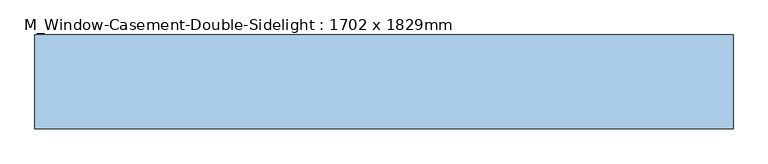
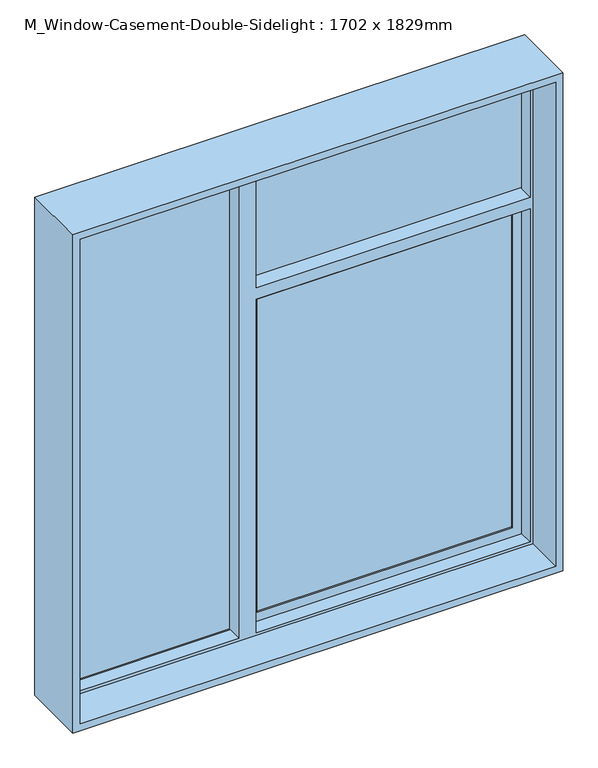
"""IFC4 building model written with IfcOpenShell, lengths in millimetres: window geometry, M_Window-Casement-Double-Sidelight : 1702 x 1829mm."""

from ifc_helpers import new_model, si_unit, frame, origin, place, context, project, spatial, polyline, outline, extrude, faceted_brep, source, transform, mapped, element, save


def m_window_casement_double_sidelight_1702_x_1829mm_c8b42c7f(model_context):
    return source(origin(), model_context, "Body", "SolidModel", [
        extrude(outline(polyline([(783.5796875, 98.4), (-102.8596875, 98.4), (-102.8596875, 111.1), (783.5796875, 111.1), (783.5796875, 98.4)])), frame((0.0, 0.0, 967.3203125), z_axis=(0.0, 0.0, 1.0), x_axis=(1.0, 0.0, 0.0)), (0.0, 0.0, 1.0), 1149.9592187),
        extrude(outline(polyline([(783.5796875, 85.7), (783.5796875, 79.35), (-102.8596875, 79.35), (-102.8596875, 85.7), (783.5796875, 85.7)])), frame((0.0, 0.0, 967.3203125), z_axis=(0.0, 0.0, 1.0), x_axis=(1.0, 0.0, 0.0)), (0.0, 0.0, 1.0), 1149.9592187),
        extrude(outline(polyline([(-195.58, 98.4), (-195.58, 92.05), (-825.5, 92.05), (-825.5, 98.4), (-195.58, 98.4)])), frame((0.0, 0.0, 935.5203125), z_axis=(0.0, 0.0, 1.0), x_axis=(1.0, 0.0, 0.0)), (0.0, 0.0, 1.0), 1767.8796875),
        extrude(outline(polyline([(-195.58, 85.7), (-195.58, 79.35), (-825.5, 79.35), (-825.5, 85.7), (-195.58, 85.7)])), frame((0.0, 0.0, 935.5203125), z_axis=(0.0, 0.0, 1.0), x_axis=(1.0, 0.0, 0.0)), (0.0, 0.0, 1.0), 1767.8796875),
        extrude(outline(polyline([(825.5, 85.7), (825.5, 79.35), (-144.78, 79.35), (-144.78, 85.7), (825.5, 85.7)])), frame((0.0, 0.0, 2201.1201563), z_axis=(0.0, 0.0, 1.0), x_axis=(1.0, 0.0, 0.0)), (0.0, 0.0, 1.0), 502.2798438),
        extrude(outline(polyline([(825.5, 98.4), (825.5, 92.05), (-144.78, 92.05), (-144.78, 98.4), (825.5, 98.4)])), frame((0.0, 0.0, 2201.1201563), z_axis=(0.0, 0.0, 1.0), x_axis=(1.0, 0.0, 0.0)), (0.0, 0.0, 1.0), 502.2798438),
        faceted_brep([(-825.5, 73.0, 2703.4), (-825.5, 114.3, 2703.4), (825.5, 114.3, 2703.4), (825.5, 73.0, 2703.4), (-144.78, 73.0, 2703.4), (-144.78, 111.1, 2703.4), (-195.58, 111.1, 2703.4), (-195.58, 73.0, 2703.4), (-815.3796875, 22.2, 2693.2796875), (-815.3796875, 73.0, 2693.2796875), (-195.58, 73.0, 2693.2796875), (-195.58, 22.2, 2693.2796875), (815.3796875, 73.0, 2693.2796875), (815.3796875, 22.2, 2693.2796875), (-134.6596875, 22.2, 2693.2796875), (-134.6596875, 73.0, 2693.2796875), (-825.5, -114.3, 2703.4), (-825.5, 22.2, 2703.4), (825.5, 22.2, 2703.4), (825.5, -114.3, 2703.4), (-850.9, 114.3, 2728.8), (-850.9, -114.3, 2728.8), (850.9, -114.3, 2728.8), (850.9, 114.3, 2728.8), (825.5, 114.3, 925.4), (825.5, 73.0, 925.4), (825.5, 73.0, 2159.1998438), (825.5, 111.1, 2159.1998438), (825.5, 111.1, 2201.1201563), (825.5, 73.0, 2201.1201563), (815.3796875, 73.0, 2201.1201563), (815.3796875, 22.2, 2201.1201563), (815.3796875, 73.0, 935.5203125), (815.3796875, 22.2, 935.5203125), (815.3796875, 22.2, 2159.1998438), (815.3796875, 73.0, 2159.1998438), (825.5, 22.2, 925.4), (825.5, -114.3, 925.4), (850.9, -114.3, 900.0), (850.9, 114.3, 900.0), (-825.5, 114.3, 925.4), (-825.5, 73.0, 925.4), (-195.58, 73.0, 925.4), (-195.58, 111.1, 925.4), (-144.78, 111.1, 925.4), (-144.78, 73.0, 925.4), (-134.6596875, 73.0, 935.5203125), (-134.6596875, 22.2, 935.5203125), (-815.3796875, 73.0, 935.5203125), (-815.3796875, 22.2, 935.5203125), (-195.58, 22.2, 935.5203125), (-195.58, 73.0, 935.5203125), (-825.5, 22.2, 925.4), (-825.5, -114.3, 925.4), (-850.9, -114.3, 900.0), (-850.9, 114.3, 900.0), (-134.6596875, 73.0, 2201.1201563), (-144.78, 73.0, 2201.1201563), (-144.78, 73.0, 2159.1998438), (-134.6596875, 73.0, 2159.1998438), (-134.6596875, 22.2, 2201.1201563), (-134.6596875, 22.2, 2159.1998438), (-144.78, 111.1, 2201.1201563), (-144.78, 111.1, 2159.1998438)], [[[0, 1, 2, 3, 4, 5, 6, 7]], [[8, 9, 10, 11]], [[12, 13, 14, 15]], [[16, 17, 18, 19]], [[20, 21, 22, 23]], [[3, 2, 24, 25, 26, 27, 28, 29]], [[13, 12, 30, 31]], [[32, 33, 34, 35]], [[19, 18, 36, 37]], [[23, 22, 38, 39]], [[25, 24, 40, 41, 42, 43, 44, 45]], [[33, 32, 46, 47]], [[48, 49, 50, 51]], [[37, 36, 52, 53]], [[39, 38, 54, 55]], [[1, 0, 41, 40]], [[12, 15, 56, 57, 4, 3, 29, 30]], [[46, 32, 35, 26, 25, 45, 58, 59]], [[41, 0, 7, 10, 9, 48, 51, 42]], [[9, 8, 49, 48]], [[17, 52, 36, 18], [13, 31, 60, 14], [33, 47, 61, 34], [49, 8, 11, 50]], [[17, 16, 53, 52]], [[22, 21, 54, 38], [16, 19, 37, 53]], [[21, 20, 55, 54]], [[20, 23, 39, 55], [2, 1, 40, 24]], [[43, 6, 5, 62, 28, 27, 63, 44]], [[6, 43, 42, 51, 50, 11, 10, 7]], [[15, 14, 60, 56]], [[47, 46, 59, 61]], [[5, 4, 57, 62]], [[45, 44, 63, 58]], [[63, 27, 26, 35, 34, 61, 59, 58]], [[28, 62, 57, 56, 60, 31, 30, 29]]]),
        extrude(outline(polyline([(2159.1998438, 825.5), (2159.1998438, -144.78), (925.4, -144.78), (925.4, 825.5), (2159.1998438, 825.5)]), holes=[polyline([(967.3203125, 783.5796875), (967.3203125, -102.8596875), (2117.2795313, -102.8596875), (2117.2795313, 783.5796875), (967.3203125, 783.5796875)])]), frame((0.0, 73.0, 0.0), z_axis=(0.0, 1.0, 0.0), x_axis=(0.0, 0.0, 1.0)), (0.0, 0.0, 1.0), 31.75),
    ])


if __name__ == "__main__":
    model = new_model("IFC4")
    model_context = context("Model", 3, world=origin())
    ifc_project = project(units=[si_unit("LENGTHUNIT", "METRE", prefix="MILLI")], contexts=[model_context])
    site = spatial("IfcSite", under=ifc_project)
    building = spatial("IfcBuilding", under=site)
    placement = place(None, origin())
    m_window_casement_double_sidelight_1702_x_1829mm_shape = m_window_casement_double_sidelight_1702_x_1829mm_c8b42c7f(model_context)
    element("IfcWindow", 1, ObjectType="M_Window-Casement-Double-Sidelight : 1702 x 1829mm", at=placement, inside=building, context=model_context, shape_type="MappedRepresentation", body=[
        mapped(m_window_casement_double_sidelight_1702_x_1829mm_shape, transform((0.0, 0.0, 0.0), x_axis=(1.0, 0.0, 0.0), y_axis=(0.0, 1.0, 0.0), z_axis=(0.0, 0.0, 1.0))),
    ])
    save(model, "model.ifc")

# Revit data of these elements
# Type "M_Window-Casement-Double-Sidelight : 1702 x 1829mm"
#   Type Mark = "18"
#   Fire Rating = "0.5h"
#   Assembly Code = "B2020100"
#   Analytic Construction = "Double glazing - domestic"
#   Window Inset [instance default] = 0' - 0.62598"
#   Wall Thickness [instance default] = 0' - 5.90551"
#   Visual Light Transmittance = 0.81
#   Transom Height Ratio = 0.3
#   Transom Height = 1' - 9.6"
#   Thermal Resistance (R) = 1.8146 (h·ft²·°F)/BTU
#   Solar Heat Gain Coefficient = 0.76
#   Side Width = 2' - 2.8"
#   Rough Width = 5' - 7.59055"
#   Rough Height = 6' - 0.59055"
#   Opening Window Width = 3' - 4.2"
#   Opening Window Height = 4' - 2.4"
#   Heat Transfer Coefficient (U) = 0.5511 BTU/(h·ft²·°F)
#   Height = 6' - 0"
#   Frame Gap 3 [instance default] = 0' - 1.65041"
#   Frame Gap 2 [instance default] = 0' - 0.62598"
#   Frame Gap 1 = 0' - 1 51/128"
#   Default Sill Height = 2' - 11.43307"
#   Width = 5' - 7"
#   Frame Material = Metal - Aluminum
#   Glass Panel Material = Glass
#   Wall Closure = (empty or 0)
# Element 1 (IfcWindow, "M_Window-Casement-Double-Sidelight : 1702 x 1829mm")
#   Wall Thickness = 0' - 9"
#   Materials on its faces: "Metal - Aluminum", "Glass"
# Materials
#   "Metal - Aluminum": class "Metal", colour RGB 247 247 247, transparency 0
#   "Glass": class "Glass", colour RGB 0 128 192, transparency 0.75, Description = "Soda Lime Glass", Cost = 0
